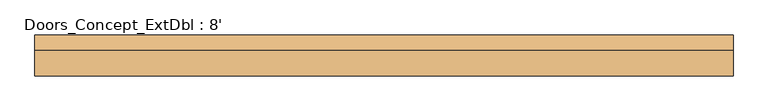
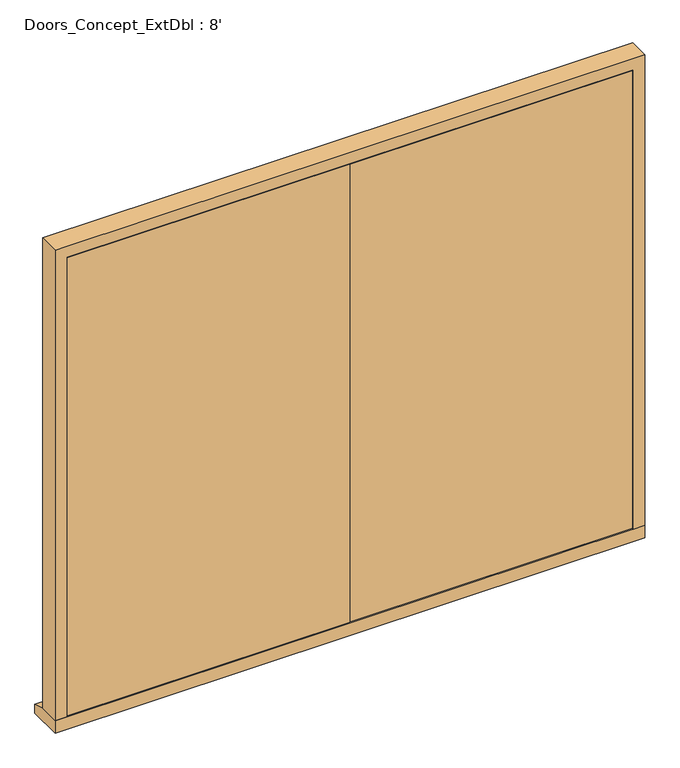
"""IFC4 building model written with IfcOpenShell, lengths in millimetres: door geometry, Doors_Concept_ExtDbl : 8'."""

from ifc_helpers import new_model, si_unit, frame, origin, place, context, project, spatial, polyline, outline, extrude, faceted_brep, source, transform, mapped, element, save


def doors_concept_extdbl_8_c180431f(model_context):
    return source(origin(), model_context, "Body", "SolidModel", [
        faceted_brep([(1148.7, 74.06, 54.5), (1219.2, 74.06, 54.5), (1219.2, -14.94, 54.5), (1170.7, -14.94, 54.5), (1170.7, 32.06, 54.5), (1148.7, 32.06, 54.5), (1148.7, 74.06, 2039.5), (-1148.7, 74.06, 2039.5), (-1148.7, 74.06, 54.5), (-1219.2, 74.06, 54.5), (-1219.2, 74.06, 2110.0), (1219.2, 74.06, 2110.0), (1219.2, -14.94, 2110.0), (-1219.2, -14.94, 2110.0), (-1219.2, -14.94, 54.5), (-1170.7, -14.94, 54.5), (-1170.7, -14.94, 2061.5), (1170.7, -14.94, 2061.5), (1170.7, 32.06, 2061.5), (-1170.7, 32.06, 2061.5), (-1170.7, 32.06, 54.5), (-1148.7, 32.06, 54.5), (-1148.7, 32.06, 2039.5), (1148.7, 32.06, 2039.5)], [[[0, 1, 2, 3, 4, 5]], [[1, 0, 6, 7, 8, 9, 10, 11]], [[2, 1, 11, 12]], [[3, 2, 12, 13, 14, 15, 16, 17]], [[4, 3, 17, 18]], [[5, 4, 18, 19, 20, 21, 22, 23]], [[0, 5, 23, 6]], [[7, 22, 21, 8]], [[8, 21, 20, 15, 14, 9]], [[13, 10, 9, 14]], [[19, 16, 15, 20]], [[12, 11, 10, 13]], [[18, 17, 16, 19]], [[6, 23, 22, 7]]]),
        extrude(outline(polyline([(1167.7, -14.94), (1.5, -14.94), (1.5, 29.06), (1167.7, 29.06), (1167.7, -14.94)])), frame((0.0, 0.0, 58.5), z_axis=(0.0, 0.0, 1.0), x_axis=(1.0, 0.0, 0.0)), (0.0, 0.0, 1.0), 2000.0),
        extrude(outline(polyline([(-1.5, -14.94), (-1167.7, -14.94), (-1167.7, 29.06), (-1.5, 29.06), (-1.5, -14.94)])), frame((0.0, 0.0, 58.5), z_axis=(0.0, 0.0, 1.0), x_axis=(1.0, 0.0, 0.0)), (0.0, 0.0, 1.0), 2000.0),
        extrude(outline(polyline([(-14.94, 0.0), (-14.94, 54.5), (74.06, 54.5), (129.06, 38.5947221), (129.06, 0.0), (-14.94, 0.0)])), frame((-1219.2, 0.0, 0.0), z_axis=(1.0, 0.0, 0.0), x_axis=(0.0, 1.0, 0.0)), (0.0, 0.0, 1.0), 2438.4),
    ])


if __name__ == "__main__":
    model = new_model("IFC4")
    model_context = context("Model", 3, world=origin())
    ifc_project = project(units=[si_unit("LENGTHUNIT", "METRE", prefix="MILLI")], contexts=[model_context])
    site = spatial("IfcSite", under=ifc_project)
    building = spatial("IfcBuilding", under=site)
    placement = place(None, origin())
    doors_concept_extdbl_8_shape = doors_concept_extdbl_8_c180431f(model_context)
    element("IfcDoor", 1, ObjectType="Doors_Concept_ExtDbl : 8'", at=placement, inside=building, context=model_context, shape_type="MappedRepresentation", body=[
        mapped(doors_concept_extdbl_8_shape, transform((0.0, 0.0, 0.0), x_axis=(1.0, 0.0, 0.0), y_axis=(0.0, 1.0, 0.0), z_axis=(0.0, 0.0, 1.0))),
    ])
    save(model, "model.ifc")

# Revit data of these elements
# Type "Doors_Concept_ExtDbl : 8'"
#   Type Mark = "53"
#   Type Comments = "External Double"
#   Operation = "DoubleDoorSingleSwing"
#   Construction Type Id = "GSP4R"
#   Keynote = "L10"
#   Analytic Construction = "1/8 in Pilkington single glazing"
#   Visual Light Transmittance = 0.9
#   Thickness = 0.144357 ft
#   Solar Heat Gain Coefficient = 0.78
#   Rough Width = 8.0 ft
#   Rough Height = 6.922572 ft
#   Heat Transfer Coefficient (U) = 3.6886 W/(m²·K)
#   FrameWidth = 0.137795 ft
#   FrameOffset - External = 0.082021 ft
#   Height = 6.922572 ft
#   Width = 8.0 ft
#   Define Thermal Properties by = 1
#   Function = 1
#   Material Door = Door - Glazing
#   Material Frame = Concept
#   Wall Closure = (empty or 0)
# Element 1 (IfcDoor, "Doors_Concept_ExtDbl : 8'")
#   Materials on its faces: "Concept", "Door - Glazing"
# Materials
#   "Door - Glazing": colour RGB 0 0 255, transparency 0.75
#   "Concept": colour RGB 128 128 255, transparency 0.5
